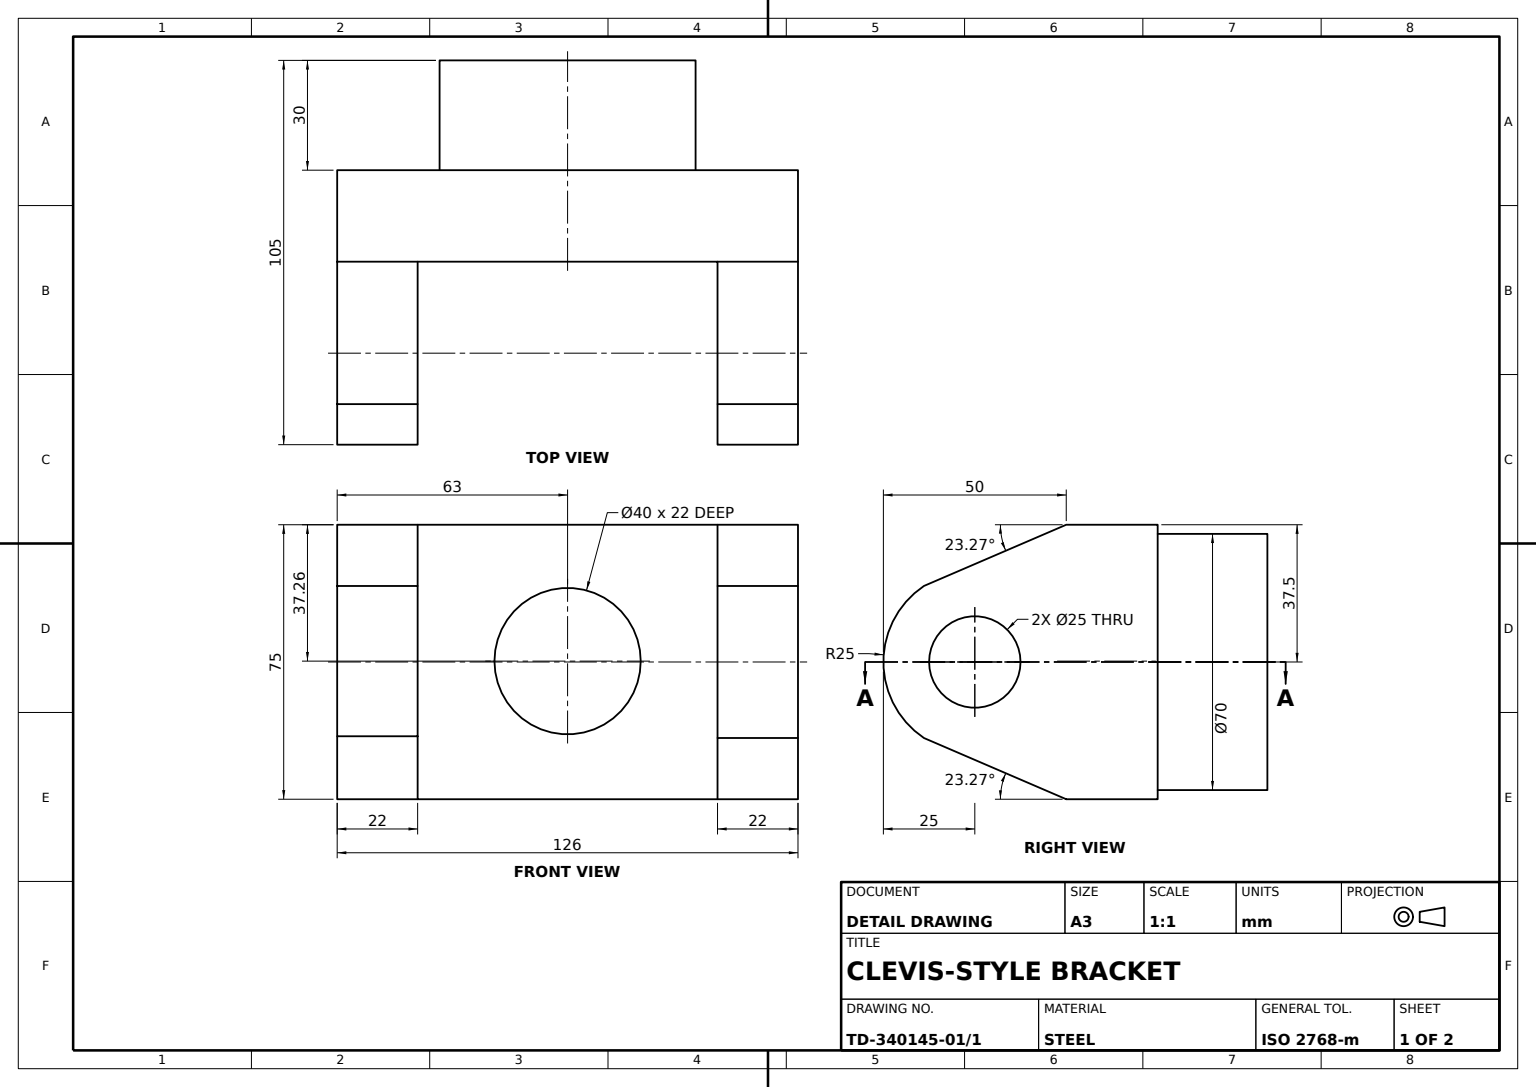
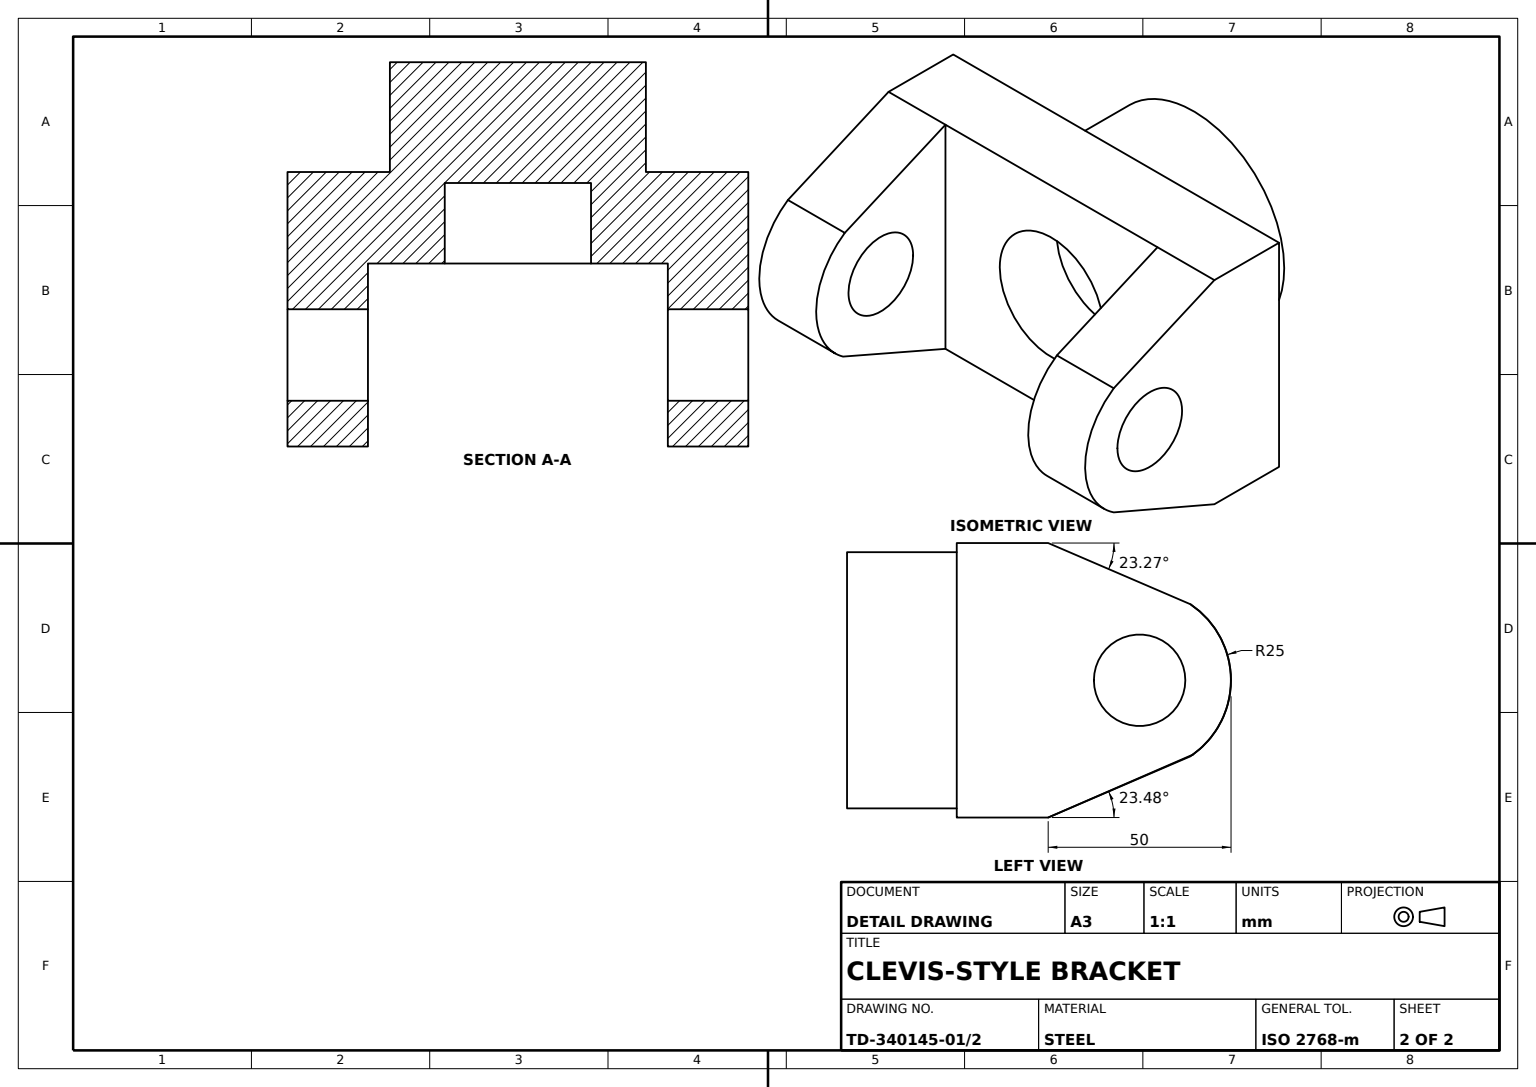
from build123d import *

# Parameters (mm, degrees)
BASE_PLATE_SKETCH_W  = 126
BASE_PLATE_SKETCH_H  = 75
BASE_PLATE_DEPTH     = 25
LUG_1_DEPTH          = 22
LUG_START            = -22
LUG_2_DEPTH          = 22
CENTRE_BORE_SKETCH_R = 20
CENTRE_BORE_40_DEPTH = 22
REAR_BOSS_SKETCH_R   = 35
REAR_BOSS_70_DEPTH   = 30
LUG_HOLE_1_SKETCH_R  = 12.5
LUG_HOLE_1_25_DEPTH  = 22
LUG_HOLE_2_SKETCH_R  = 12.5
LUG_HOLE_2_25_DEPTH  = 22


with BuildPart() as part:
    # Base Plate Sketch → Base Plate (new body)
    with BuildSketch(Plane.XY):
        with Locations((63, 37.5)):
            Rectangle(BASE_PLATE_SKETCH_W, BASE_PLATE_SKETCH_H)
    extrude(amount=BASE_PLATE_DEPTH)

    # Lug 1 Sketch → Lug 1 (add)
    with BuildSketch(Plane(origin=(126, 0, 0), x_dir=(0, 0, -1), z_dir=(1, 0, 0))):
        with BuildLine():
            Line((-25, 75), (-25, 0))
            Line((-25, 0), (-63.918991375, 16.733159145))
            ThreePointArc((-63.918991375, 16.733159145), (-75, 37.5), (-63.918991375, 58.266840855))
            Line((-63.918991375, 58.266840855), (-25, 75))
        make_face()
    extrude(amount=-LUG_1_DEPTH)

    # Lug 2 Sketch → Lug 2 (add)
    with BuildSketch(Plane.ZY.offset(LUG_START)):
        with BuildLine():
            Line((25, 75), (25, 0))
            Line((25, 0), (64.599836332, 17.206040823))
            ThreePointArc((64.599836332, 17.206040823), (74.996563929, 37.914477664), (63.918991375, 58.266840855))
            Line((63.918991375, 58.266840855), (25, 75))
        make_face()
    extrude(amount=LUG_2_DEPTH)

    # Centre Bore Sketch → Centre Bore Ø40 (cut)
    with BuildSketch(Plane.XY.offset(25)):
        with Locations((63, 37.736440839)):
            Circle(CENTRE_BORE_SKETCH_R)
    extrude(amount=-CENTRE_BORE_40_DEPTH, mode=Mode.SUBTRACT)

    # Rear Boss Sketch → Rear Boss Ø70 (add)
    with BuildSketch(Plane(origin=(0, 0, 0), x_dir=(-1, 0, 0), z_dir=(0, 0, -1))):
        with Locations((-63, 37.5)):
            Circle(REAR_BOSS_SKETCH_R)
    extrude(amount=REAR_BOSS_70_DEPTH)

    # Lug Hole 1 Sketch → Lug Hole 1 Ø25 (cut)
    with BuildSketch(Plane.ZY):
        with Locations((50, 37.5)):
            Circle(LUG_HOLE_1_SKETCH_R)
    extrude(amount=-LUG_HOLE_1_25_DEPTH, mode=Mode.SUBTRACT)

    # Lug Hole 2 Sketch → Lug Hole 2 Ø25 (cut)
    with BuildSketch(Plane(origin=(126, 0, 0), x_dir=(0, 0, -1), z_dir=(1, 0, 0)).offset(LUG_START)):
        with Locations(Location((-50, 37.5, 0), (0, 0, 180))):
            Circle(LUG_HOLE_2_SKETCH_R)
    extrude(amount=LUG_HOLE_2_25_DEPTH, mode=Mode.SUBTRACT)


solid = part.part
